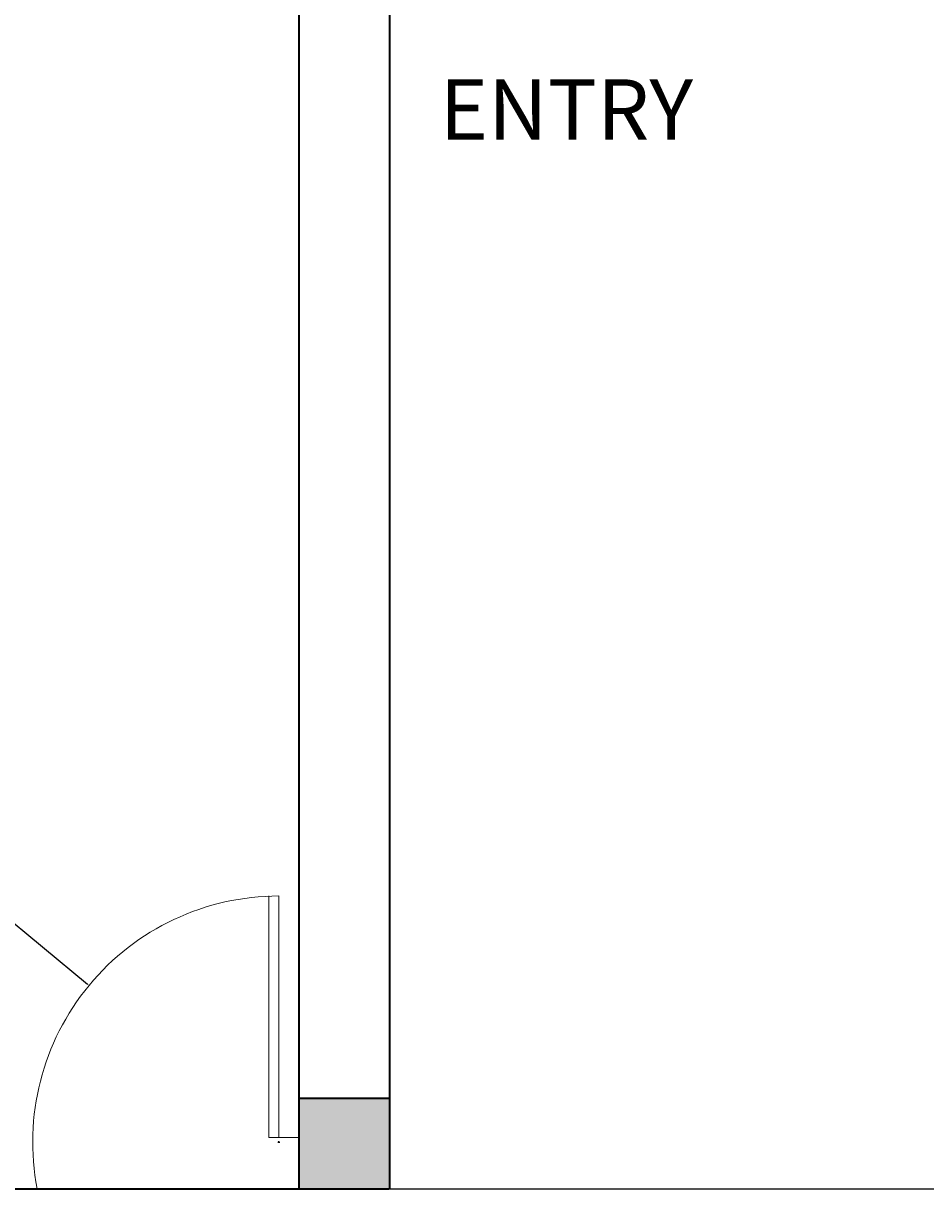
# Model space of a CAD drawing. Units: inches. Extents: x 5 to 421, y -617 to 43.
# Tile 4 of 15: x 133 to 223, y -585 to -469. Entities that reach past the tile are written whole.
import ezdxf

# ---------------------------------------------------------------- set-up
doc = ezdxf.new("R2010")
doc.units = ezdxf.units.IN
doc.header["$MEASUREMENT"] = 0
for name, color, linetype, lineweight in [('A-ANNO-DIMS', 2, 'Continuous', 18), ('A-ANNO-TEXT', 7, 'Continuous', 18), ('A-SITE-GATE', 3, 'Continuous', 20), ('A-WALL', 7, 'Continuous', 35)]:
    doc.layers.add(name, color=color, linetype=linetype, lineweight=lineweight)
doc.layers.add('A-WALL-PATT', color=251, linetype='Continuous', lineweight=13, true_color=0x636466)
doc.styles.get("Standard").update_dxf_attribs({"font": 'arial.ttf'})
doc.dimstyles.get("Standard").update_dxf_attribs({"dimtxt": 0.18, "dimasz": 0.18, "dimexe": 0.18, "dimexo": 0.0625, "dimgap": 0.09, "dimtad": 0, "dimtih": 1, "dimtoh": 1, "dimdec": 0, "dimzin": 0, "dimdsep": 46, "dimlunit": 3, "dimtxsty": 'Standard', "dimcen": 0.09, "dimadec": 0, "dimazin": 0, "dimtfac": 1, "dimtdec": 0, "dimtofl": 0, "dimtmove": 0, "dimatfit": 3, "dimfxl": 1, "dimtolj": 1, "dimtzin": 0, "dimarcsym": 0})

# ---------------------------------------------------------------- blocks, each defined once
blk = doc.blocks.new('*D55')
at = {"layer": 'A-ANNO-DIMS', "color": 0, "lineweight": -2, "transparency": 16777216}
for p, q in [((370.48, 10.88), (420.4, 10.88)), ((420.22, 10.7), (420.22, -286.69)), ((420.22, -584.44), (420.22, -287.05)), ((169.48, -584.62), (420.4, -584.62))]:
    blk.add_line(p, q, dxfattribs=at)
at = {"layer": 'A-ANNO-DIMS', "color": 0, "transparency": 16777216}
for points in [[(420.19, 10.7), (420.25, 10.7), (420.22, 10.88)], [(420.19, -584.44), (420.25, -584.44), (420.22, -584.62)]]:
    blk.add_solid(points, dxfattribs=at)
at = {"layer": 'Defpoints', "color": 0, "transparency": 16777216}
for p in [(370.42, 10.88), (169.42, -584.62), (420.22, -584.62)]:
    blk.add_point(p, dxfattribs=at)
at = {"layer": 'A-ANNO-DIMS', "color": 0, "transparency": 16777216, "insert": (420.22, -286.87), "char_height": 0.18, "attachment_point": 5}
blk.add_mtext('\\A1;595.5', dxfattribs=at)
blk = doc.blocks.new('*D82')
at = {"layer": 'A-ANNO-DIMS', "color": 0, "lineweight": -2, "transparency": 16777216}
for p, q in [((128.08, -555.09), (128.26, -555.09)), ((128.26, -555.09), (139.43, -564.32)), ((158.33, -579.99), (158.51, -579.99)), ((158.42, -580.08), (158.42, -579.9))]:
    blk.add_line(p, q, dxfattribs=at)
at = {"layer": 'A-ANNO-DIMS', "color": 0, "transparency": 16777216}
blk.add_solid([(139.45, -564.29), (139.41, -564.34), (139.57, -564.43)], dxfattribs=at)
at = {"layer": 'Defpoints', "color": 0, "transparency": 16777216}
for p in [(139.57, -564.43), (158.42, -579.99)]:
    blk.add_point(p, dxfattribs=at)
at = {"layer": 'A-ANNO-DIMS', "color": 0, "transparency": 16777216, "insert": (127.6, -555.09), "char_height": 0.18, "attachment_point": 5}
blk.add_mtext('\\A1;R24.44', dxfattribs=at)

msp = doc.modelspace()

# ---------------------------------------------------------------- hatches: boundary and pattern name
at = {"layer": 'A-WALL-PATT'}
h = msp.add_hatch(color=256, dxfattribs=at)
h.dxf.hatch_style = 1
h.paths.add_polyline_path([(46.4196, -88.1188), (37.4196, -88.1188), (37.4196, -166.6119), (46.4196, -166.6119), (46.4196, -122.6188), (135.4196, -122.6188), (135.4196, -120.3688), (135.4196, -118.1188), (46.4196, -118.1188)])
h.paths.add_polyline_path([(82.4196, 10.8812), (37.4196, 10.8812), (37.4196, -28.1188), (46.4196, -28.1188), (46.4196, 1.8812), (82.4196, 1.8812)])
h.paths.add_polyline_path([(215.5968, 10.8812), (142.4196, 10.8812), (142.4196, 1.8812), (178.4196, 1.8812), (178.4196, -118.1188), (175.4196, -118.1188), (175.4196, -122.6188), (182.9196, -122.6188), (182.9196, -80.6188), (211.9196, -80.6188), (211.9196, -78.3688), (211.9196, -76.1188), (182.9196, -76.1188), (182.9196, 1.8812), (215.5968, 1.8812)])
h.paths.add_polyline_path([(274.4196, 10.8812), (239.5968, 10.8812), (239.5968, 1.8812), (242.9196, 1.8812), (242.9196, -76.1188), (239.9196, -76.1188), (239.9196, -80.6188), (242.9196, -80.6188), (242.9196, -83.6188), (247.4196, -83.6188), (247.4196, 1.8812), (274.4196, 1.8812)])
h.paths.add_polyline_path([(370.4196, 10.8812), (334.4196, 10.8812), (334.4196, 1.8812), (361.4196, 1.8812), (361.4196, -28.1188), (370.4196, -28.1188)])
h.paths.add_polyline_path([(370.4196, -88.1188), (361.4196, -88.1188), (361.4196, -118.1188), (247.4196, -118.1188), (247.4196, -115.1188), (242.9196, -115.1188), (242.9196, -118.1188), (220.4196, -118.1188), (220.4196, -158.6188), (224.9196, -158.6188), (224.9196, -122.6188), (326.9196, -122.6188), (326.9196, -170.7662), (331.4196, -170.7662), (331.4196, -122.6188), (370.4196, -122.6188)])
h.paths.add_polyline_path([(388.4196, -122.6188), (388.4196, -118.1188), (379.4196, -118.1188), (379.4196, -122.6188), (379.4196, -154.8688), (388.4196, -154.8688)])
h.paths.add_polyline_path([(388.4196, -214.8688), (379.4196, -214.8688), (379.4196, -247.1188), (388.4196, -247.1188)])
h.paths.add_polyline_path([(371.0265, -242.6188), (331.4196, -242.6188), (331.4196, -239.6188), (326.9196, -239.6188), (326.9196, -242.6188), (224.9196, -242.6188), (224.9196, -206.6188), (220.4196, -206.6188), (220.4196, -343.6188), (224.9196, -343.6188), (229.4196, -343.6188), (229.4196, -247.1188), (261.5265, -247.1188), (261.5265, -276.1188), (263.7765, -276.1188), (266.0265, -276.1188), (266.0265, -247.1188), (362.0265, -247.1188), (362.0265, -265.1188), (371.0265, -265.1188), (371.0265, -247.1188)])
h.paths.add_polyline_path([(371.0265, -289.1188), (362.0265, -289.1188), (362.0265, -307.1188), (266.0265, -307.1188), (266.0265, -304.1188), (261.5265, -304.1188), (261.5265, -307.1188), (261.5265, -311.6188), (362.0265, -311.6188), (362.0265, -353.6188), (371.0265, -353.6188)])
h.paths.add_polyline_path([(371.0265, -413.6188), (362.0265, -413.6188), (362.0265, -455.6188), (325.7231, -455.6188), (325.7231, -464.6188), (361.4196, -464.6188), (371.0265, -464.6188)])
h.paths.add_polyline_path([(265.7231, -455.6188), (229.4196, -455.6188), (229.4196, -383.6188), (220.4196, -383.6188), (220.4196, -386.6188), (207.4649, -386.6188), (207.4649, -395.6188), (220.4196, -395.6188), (220.4196, -455.6188), (216.0568, -455.6188), (216.0568, -464.6188), (265.7231, -464.6188)])
h.paths.add_polyline_path([(169.4196, -386.6188), (137.9196, -386.6188), (137.9196, -395.6188), (160.4196, -395.6188), (160.4196, -424.2032), (169.4196, -424.2032)])
h.paths.add_polyline_path([(169.4196, -453.7423), (160.4196, -453.7423), (160.4196, -464.6188), (169.4196, -464.6188)])
h.paths.add_polyline_path([(46.4196, -575.6188), (37.4196, -575.6188), (37.4196, -584.6188), (46.4196, -584.6188)])
h.paths.add_polyline_path([(169.4196, -575.6188), (160.4196, -575.6188), (160.4196, -579.5504), (160.4196, -584.6188), (169.4196, -584.6188)])
h.paths.add_polyline_path([(46.4196, -226.6119), (37.4196, -226.6119), (37.4196, -292.8008), (46.4196, -292.8008)])
h.paths.add_polyline_path([(46.4196, -352.8008), (37.4196, -352.8008), (37.4196, -395.6188), (77.9196, -395.6188), (77.9196, -386.6188), (46.4196, -386.6188)])

# ---------------------------------------------------------------- linework, layer by layer
at = {"layer": 'A-SITE-GATE'}
for p, q in [((157.4196, -579.5504), (157.4196, -555.5504)), ((158.4196, -579.5504), (158.4196, -555.5504)), ((160.4196, -579.5504), (157.4196, -579.5504))]:
    msp.add_line(p, q, dxfattribs=at)
msp.add_arc((158.4196, -579.9922), 24.4419, 90, 190.911328, dxfattribs=at)
at = {"layer": 'A-WALL'}
for p, q in [((169.4196, -386.6188), (169.4196, -584.6188)), ((160.4196, -395.6188), (160.4196, -584.6188)), ((160.4196, -575.6188), (169.4196, -575.6188)), ((37.4196, -584.6188), (169.4196, -584.6188))]:
    msp.add_line(p, q, dxfattribs=at)

# ---------------------------------------------------------------- texts
at = {"layer": 'A-ANNO-TEXT', "insert": (174.3832, -474.4525), "char_height": 6, "attachment_point": 1}
msp.add_mtext('ENTRY', dxfattribs=at)

# ---------------------------------------------------------------- dimensions: what is measured, and where the dimension line sits
at = {"layer": 'A-ANNO-DIMS'}
dim = msp.add_linear_dim(base=(420.2196, -584.6188), p1=(370.4196, 10.8812), p2=(169.4196, -584.6188), angle=90, dimstyle='Standard', override={"dimdec": 1, "dimlfac": 1, "dimrnd": 0, "dimzin": 0, "dimdsep": 46, "dimlunit": 2}, dxfattribs=at)
dim.commit()
dim.dimension.update_dxf_attribs({"geometry": '*D55', "text_midpoint": (420.2196, -286.8688)})
dim = msp.add_radius_dim(center=(158.4196, -579.9922), mpoint=(139.5717, -564.4307), dimstyle='Standard', override={"dimdec": 2, "dimlfac": 1, "dimrnd": 0, "dimzin": 0, "dimdsep": 46, "dimlunit": 2}, dxfattribs=at)
dim.commit()
dim.dimension.update_dxf_attribs({"geometry": '*D82', "text_midpoint": (127.6034, -555.0938), "dimtype": 164})

doc.saveas('drawing.dxf')
